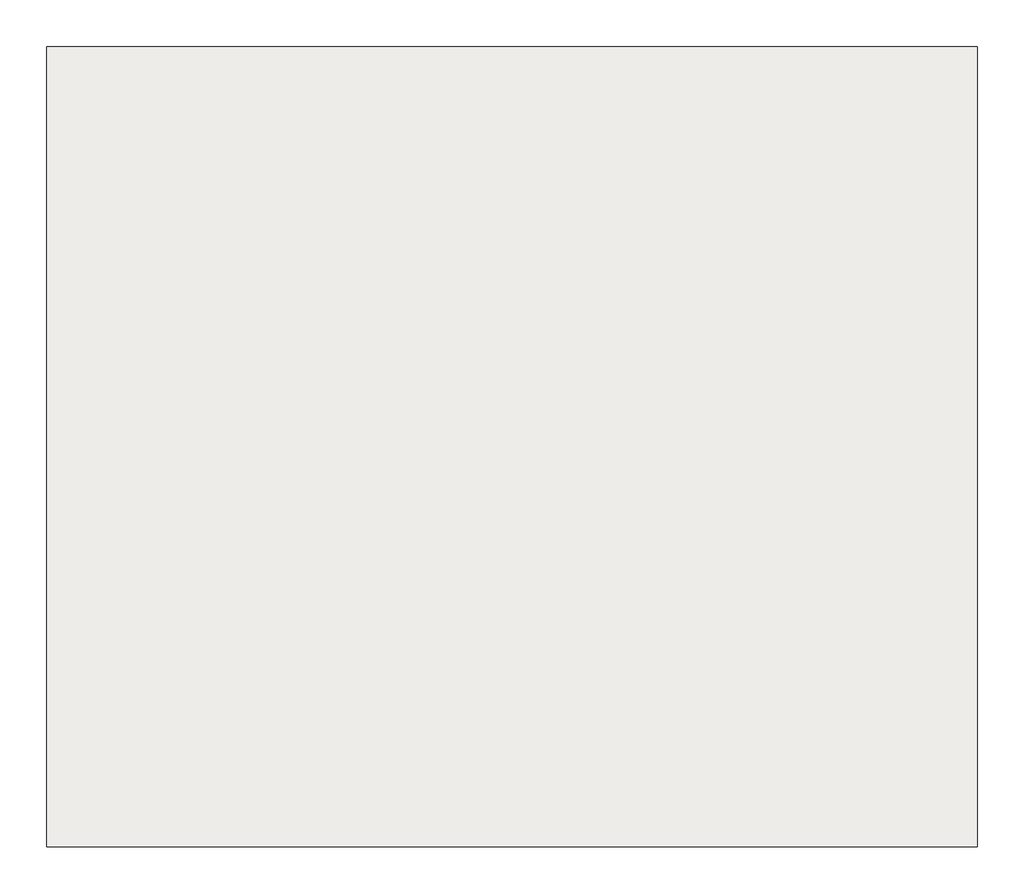
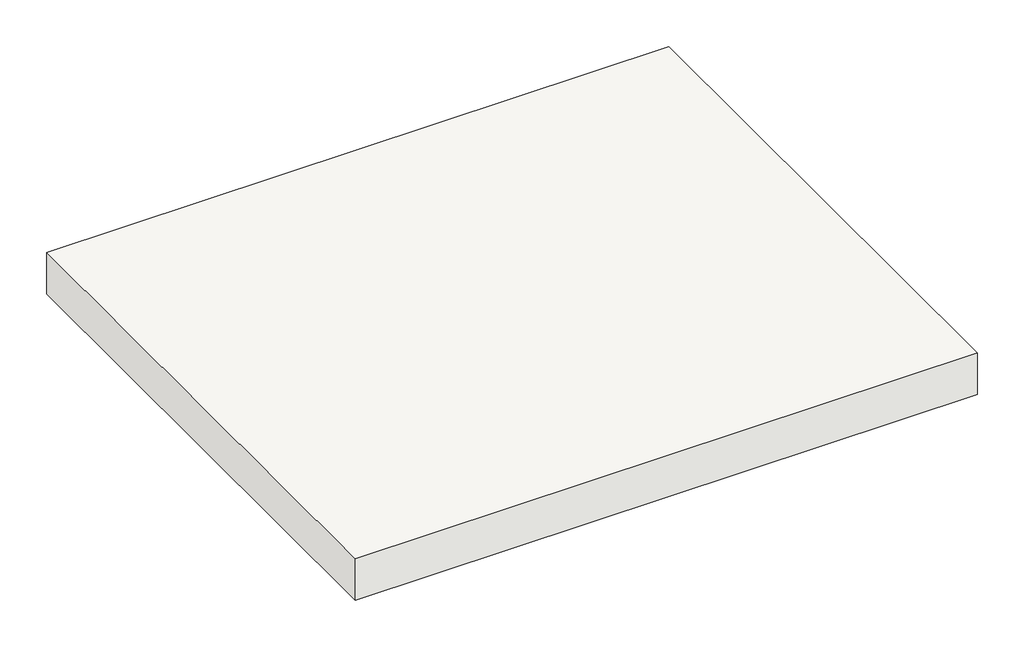
# One storey: 1 slab.
"""IFC4 building model written with IfcOpenShell, lengths in millimetres."""

from ifc_helpers import new_model, si_unit, frame, origin, place, context, project, spatial, polyline, outline, extrude, element, save

model = new_model("IFC4")

# Units and contexts
model_context = context("Model", 3, world=origin())
ifc_project = project(units=[si_unit("LENGTHUNIT", "METRE", prefix="MILLI")], contexts=[model_context])

# Site, building, storey
site = spatial("IfcSite", under=ifc_project)
building = spatial("IfcBuilding", under=site)
storey = spatial("IfcBuildingStorey", under=building, Elevation=4876.8)

# Slab
placement = place(None, origin())
element("IfcSlab", 1, ObjectType="SLAB FLOOR", at=placement, inside=storey, context=model_context, shape_type="SweptSolid", body=[
    extrude(outline(polyline([(-4410.4677418, -371.3477572), (-4410.4677418, 2061.9722428), (-1580.4996772, 2061.9722428), (-1580.4996772, -371.3477572), (-4410.4677418, -371.3477572)])), frame((0.0, 0.0, 4876.8), z_axis=(0.0, 0.0, 1.0), x_axis=(1.0, 0.0, 0.0)), (0.0, 0.0, 1.0), 199.9488),
])

save(model, "model.ifc")

# Revit data of these elements
# Type "SLAB FLOOR"
#   Layers, outside or top first: 199.949 mm "Concrete, Precast" (function 1)
# Element 1 (IfcSlab, "SLAB FLOOR")
#   built-in parameter 1001955 = 3.14159 (stored number, unit not read)
#   Height Offset From Level = 199.949 mm
#   built-in parameter 1001954 = 1
#   Phase Created = New Construction
#   Materials on its faces: "Concrete, Precast"
# Materials
#   "Concrete, Precast": class "Concrete", colour RGB 192 192 192, transparency 0, Description = "Precast concrete", Cost = 0
